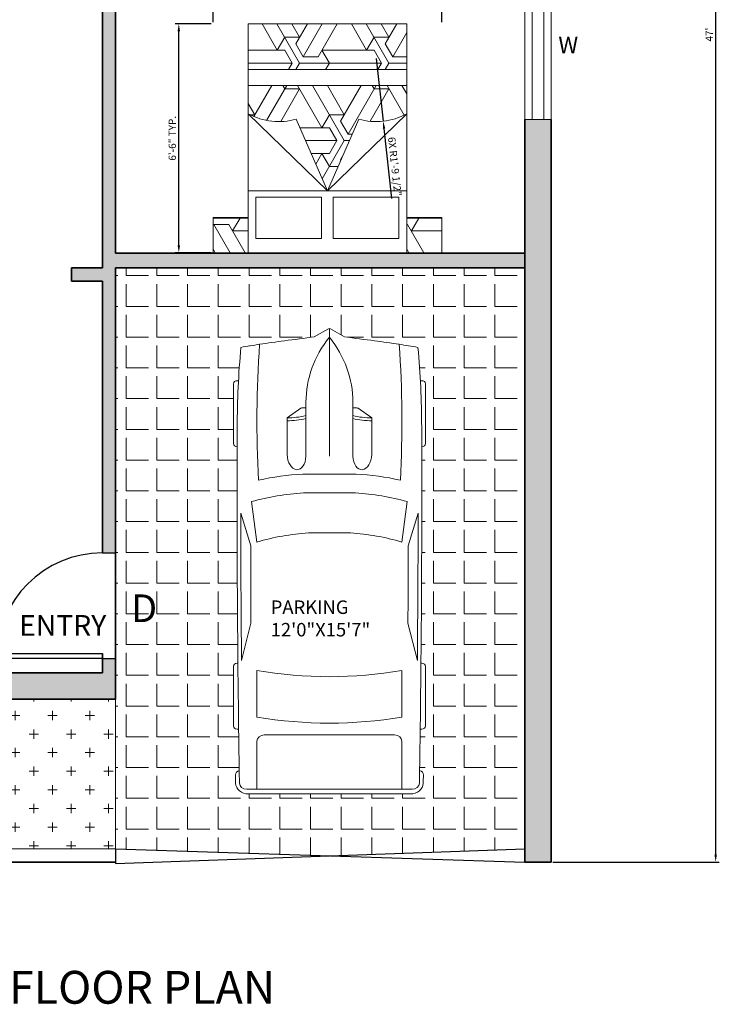
# Model space of a CAD drawing. Units: inches. Extents: x 1878 to 2382, y 1889 to 2524.
# Tile 1 of 2: x 2143 to 2382, y 1889 to 2225. Entities that reach past the tile are written whole.
import ezdxf

# ---------------------------------------------------------------- set-up
doc = ezdxf.new("R2010")
doc.units = ezdxf.units.IN
for name, color, linetype, lineweight in [('A-ANNO-DIMS', 2, 'Continuous', 18), ('A-ANNO-TEXT', 7, 'Continuous', 18), ('A-ANNO-TITL', 7, 'Continuous', 30), ('A-AREA-IDEN', 7, 'Continuous', 18), ('A-DOOR', 4, 'Continuous', 25), ('A-FLOR-PATT', 252, 'Continuous', 13), ('A-FURN', 8, 'Continuous', 18), ('A-FURN-PATT', 252, 'Continuous', 13), ('A-SITE-GATE', 1, 'Continuous', 25), ('A-SITE-VEHI', 8, 'Continuous', 18), ('A-WALL', 7, 'Continuous', 35), ('A-WALL-PATT', 251, 'Continuous', 13), ('L-PLNT', 3, 'Continuous', 18), ('L-PLNT-PATT', 3, 'Continuous', 13), ('windows', 5, 'Continuous', 18)]:
    doc.layers.add(name, color=color, linetype=linetype, lineweight=lineweight)
doc.styles.get("Standard").update_dxf_attribs({"font": 'arial.ttf'})
doc.dimstyles.new('ISO-25', dxfattribs={"dimtxt": 2.5, "dimasz": 2.5, "dimexe": 1.25, "dimexo": 0.625, "dimtad": 1, "dimlunit": 3, "dimtxsty": 'Standard', "dimcen": 2.5, "dimadec": 0, "dimazin": 0, "dimtfac": 1, "dimtmove": 0, "dimatfit": 3, "dimfxl": 1, "dimarcsym": 0})

# ---------------------------------------------------------------- blocks, each defined once
blk = doc.blocks.new('*D15')
at = {"layer": 'A-ANNO-DIMS', "color": 0, "lineweight": -2, "transparency": 16777216}
for p, q in [((2324.866440692248, 2501.568149098086), (2381.60236904706, 2501.568149098086)), ((2380.35236904706, 2499.068149098085), (2380.35236904706, 1940.068149098086)), ((2324.866440692248, 1937.568149098086), (2381.60236904706, 1937.568149098086))]:
    blk.add_line(p, q, dxfattribs=at)
at = {"layer": 'A-ANNO-DIMS', "color": 0, "transparency": 16777216}
for points in [[(2379.935702380393, 2499.068149098085), (2380.769035713727, 2499.068149098085), (2380.35236904706, 2501.568149098086)], [(2379.935702380393, 1940.068149098086), (2380.769035713727, 1940.068149098086), (2380.35236904706, 1937.568149098086)]]:
    blk.add_solid(points, dxfattribs=at)
at = {"layer": 'Defpoints', "color": 0, "transparency": 16777216}
for p in [(2324.241440692248, 2501.568149098086), (2324.241440692248, 1937.568149098086), (2380.35236904706, 1937.568149098086)]:
    blk.add_point(p, dxfattribs=at)
at = {"layer": 'A-ANNO-DIMS', "color": 0, "transparency": 16777216, "insert": (2378.47736904706, 2219.568149098085), "char_height": 2.5, "attachment_point": 5, "rotation": 90}
blk.add_mtext("47'", dxfattribs=at)
blk = doc.blocks.new('*U2')
for p, q in [((0, 0), (-1e-16, -3.999999999999999)), ((36, -4e-16), (36, -3.999999999999999))]:
    blk.add_line(p, q)
blk.add_lwpolyline([(0, 0), (5.2e-15, 36), (1.750000000000006, 36), (1.749999999999998, -7e-16)], close=True)
blk.add_arc((0, 0), 36, 0, 90)
blk = doc.blocks.new('*U17')
for p, q in [((21.10406751471477, 37.40863046792069), (21.10406751471477, 36.83230215753705)), ((46.55368679439944, 38.88847654282876), (22.35054758993934, 38.88847654282876)), ((47.80016686962392, 37.39011648242055), (47.80016686962392, 37.40863046792069)), ((87.98532186932616, 31.87120872459877), (74.75900729854769, 35.92175679182955)), ((135.4513231603356, 37.07354110333037), (135.4513231603356, 37.40863046792069)), ((136.6978032355602, 38.88847654282876), (160.90094244002, 38.88847654282867)), ((162.1474225152445, 37.40863046792049), (162.1474225152445, 36.77402019194128)), ((134.313356548143, 35.6043097713567), (119.2882629232503, 31.77757799177584)), ((186.4728846989705, -33.49860931502491), (186.4728846989718, 33.49860931502465)), ((188.3990091454065, -32.75868627757393), (188.3990091454077, 32.75868627757058)), ((70.0302824853563, 31.53613089391356), (86.40615155322342, 29.35124891408057)), ((138.4228833961707, 29.35124891408074), (157.2465674415997, 29.35124891408074)), ((186.4728846989718, 29.35124891408083), (167.0083537481071, 29.35124891408083)), ((164.515393597658, 26.39155676426461), (164.5153935976578, -26.39155676426503)), ((32.26591480791686, 11.62530558863241), (36.12873726252356, 17.16961494239206)), ((36.12873726252356, 17.16961494239206), (50.93891189819171, 17.16961494239206)), ((29.77279020470884, 9.505833383620029), (51.68362801571248, 9.505833383620029)), ((32.12291633764599, 9.505833383620029), (32.12291633764599, 11.15369945057711)), ((58.9167604809788, -10.77488335095668), (58.9167604809788, 10.77488335095617)), ((66.55009204259746, -10.5288681329018), (66.55009204259746, 10.52886813290129)), ((82.73706193978568, 8.496039918672748), (82.73706193978568, -8.49603991867258)), ((186.4728846989718, -10.5288681329018), (186.4728846989718, 10.52886813290129)), ((3.266462181856987, 6.128290093440767), (0.1022408397004821, 0.4060708604429806)), ((-4.43e-14, -2.558e-13), (51.68362801571248, -2.558e-13)), ((0.1022408397004821, -0.4060708604432933), (3.266462181856987, -6.128290093441194)), ((29.77279020470884, -9.50583338362054), (51.68362801571248, -9.50583338362054)), ((32.12291633764599, -9.50583338362054), (32.12291633764599, -11.15369945057762)), ((32.26591480791686, -11.62530558863292), (36.12873726252356, -17.16961494239257)), ((36.12873726252356, -17.16961494239257), (50.93891189819171, -17.16961494239257)), ((86.40615155322318, -29.35124891408145), (70.03028248535594, -31.53613089391442)), ((87.98532186932607, -31.87120872459903), (74.7590072985476, -35.92175679182964)), ((134.3133565481428, -35.60430977135721), (119.2882629232503, -31.77757799177618)), ((157.2465674415997, -29.35124891408117), (138.4228833961707, -29.35124891408126)), ((167.008353748107, -29.35124891408126), (186.4728846989707, -29.35124891408108)), ((21.10406751471477, -37.4086304679212), (21.10406751471477, -36.83230215753756)), ((46.55368679439944, -38.88847654282927), (22.35054758993934, -38.88847654282927)), ((47.80016686962392, -37.39011648242107), (47.80016686962392, -37.4086304679212)), ((135.4513231603355, -37.07354110333088), (135.4513231603355, -37.4086304679212)), ((136.6978032355602, -38.88847654282927), (160.9009424400199, -38.88847654282918)), ((162.1474225152445, -37.408630467921), (162.1474225152445, -36.77402019194179))]:
    blk.add_line(p, q)
for centre, major_axis, ratio, start_param, end_param in [((41.19115208863305, -490.8631038926156), (1.294e-13, 528.2339998381949), 0.8423038695439741, 0.0028100083536837, 0.0755983031096952), ((22.35054758993934, 37.40863046792072), (2.08e-14, -1.479846074908118), 0.842303869543976, 3.141592653589776, 4.712388980384677), ((64.48199294511879, -10555.61767587835), (1.907644e-10, 10593.02630634627), 0.842303869543847, -0.0133969486112073, 0.0027970409639888), ((46.55368679439944, 37.40863046792072), (2.2e-14, 1.479846074908118), 0.8423038695439758, -1.570796326794884, 1.73e-14), ((64.4819929449925, -10555.61767590795), (1.9177683e-09, -10591.54646030096), 0.8423038695482963, 3.133765086725325, 3.140440689641252), ((136.6978032355602, 37.40863046792072), (2.357e-13, -1.479846074908118), 0.842303869543976, 3.141592653589603, 4.712388980384554), ((160.90094244002, 37.40863046792052), (5.59e-14, 1.479846074908118), 0.842303869543976, -1.570796326794865, 4.44e-14), ((180.6280394947615, 35.8381667808375), (7.4e-14, 2.219769112362114), 0.8423038695439693, -0.0130174256259048, 1.249894140392862), ((64.48199294754608, -10556.35759891604), (1.349839377e-06, 10595.3130398087), 0.8423038681351469, -0.0133969484821159, -0.0130174254969711), ((183.9799245485226, 33.49860931502124), (3e-16, -2.959692149816168), 0.8423038695439952, 1.570796326796048, 3.128195704978389), ((183.9799245485216, 32.75868627756583), (8.56e-14, -5.246425615115243), 0.8423038695439737, 1.570796326795794, 3.128195704978164), ((266.0300214172791, -27.52442688366631), (1.966072e-10, 313.3077612809058), 0.8423038695435284, 1.367075990158062, 1.391760499156098), ((95.78879860270445, -3666.353346297651), (1.949864e-10, -3698.236159209632), 0.8423038695446962, 3.134048706297306, 3.14409775411291), ((259.1750197310735, -27.52442688366614), (1.506617e-10, -305.3028914627677), 0.8423038695443789, 4.528606069860317, 4.561837674556238), ((37.47375371777758, -593.9621830607928), (6.21e-14, -623.32820996736), 0.8423038695439826, 3.09604606856106, 3.200911180495224), ((134.4003789125686, 5.387441675477674), (4.276e-13, -89.7774543484738), 0.84230386954398, 4.44948196380473, 4.652344057257214), ((135.2911776514449, 5.387441675478555), (2.2715e-12, 81.77258453065997), 0.8423038695439563, 1.245306111696802, 1.507880129813836), ((149.595361812917, 2.799442537139299), (8.561e-13, -79.57966406425402), 0.842303869543983, 4.372215489277867, 4.640744122441986), ((17.08207736189386, -1.421e-13), (6.87e-14, 147.0179238898305), 0.8423038695439764, 4.511394369635731, 4.913383591133647), ((35.90576140732288, -1.421e-13), (6.87e-14, 147.0179238898305), 0.8423038695439764, 4.511394369635731, 4.913383591133647), ((167.0083537481071, 26.39155676426464), (1.394e-13, 2.959692149816236), 0.842303869543976, 5.55e-14, 1.57079632679492), ((-204.4946649195746, 52.39684969293512), (4.12053e-11, -250.9602162198571), 0.8423038695441164, 1.385369446298923, 1.434372047871027), ((13.03653510440275, 17.00972444508943), (1.2303e-12, 27.41599049210566), 0.8423038695439277, 4.435146050259648, 4.718221029521873), ((14.20086229321332, 17.00972444508943), (1.2303e-12, 27.41599049210566), 0.8423038695439277, 4.435146050259648, 4.718221029521873), ((50.7902773840875, 13.33772416300607), (6.340077547122382, -0.356608581037027), 0.6038335755719145, -1.39555193967809, 1.581314658479915), ((29.77279020470884, -46.66302566589627), (5.12e-14, 56.16885904951626), 0.842303869543976, 7e-16, 0.5903187773915901), ((32.74615637525823, 11.15369945057713), (1.313e-13, 0.7399230374541176), 0.8423038695439091, 0.8797135699495516, 1.570796326795045), ((0.6232400376122422, -1.421e-13), (1e-16, -0.7399230374541245), 0.842303869543842, 4.131459131953847, 5.293318828815531), ((29.77279020470884, 46.66302566589578), (4.004e-13, 56.16885904951626), 0.8423038695439734, 2.55127387619821, 3.141592653589801), ((-204.4946649195746, -52.39684969293552), (4.02945e-11, 250.9602162198562), 0.8423038695441192, -1.43437204787103, -1.385369446298926), ((32.74615637525823, -11.1536994505777), (1.3e-13, -0.7399230374541176), 0.8423038695439093, 4.712388980384541, 5.403471737230034), ((13.03653510440275, -17.00972444508983), (1.2568e-12, -27.41599049210552), 0.8423038695439318, 1.564964277657711, 1.848039256919935), ((14.20086229321332, -17.00972444508983), (1.2568e-12, -27.41599049210552), 0.8423038695439318, 1.564964277657711, 1.848039256919935), ((134.4003789125684, -5.387441675478584), (4.2949e-12, -89.77745434847827), 0.8423038695439354, -1.510751403667474, -1.307889310215002), ((135.2911776514465, -5.387441675480715), (3.2038e-12, -81.77258453066244), 0.8423038695439492, -1.50788012981387, -1.245306111696839), ((149.5953618129329, -2.799442537137565), (4.0897e-12, -79.57966406427697), 0.8423038695439419, -1.499151468852248, -1.230622835688196), ((259.1750197310694, 27.52442688365929), (1.08535e-11, 305.3028914629043), 0.8423038695439974, 1.721347632622872, 1.754579237318777), ((167.008353748107, -26.39155676426503), (1.02e-14, -2.959692149816192), 0.8423038695439885, 4.712388980384686, 6.283185307179581), ((266.0300214172791, 27.52442688366566), (8.75241e-11, 313.3077612806533), 0.8423038695441819, 1.749832154434603, 1.774516663432659), ((37.47375371777847, 593.9621830607904), (1.1693e-12, -623.3282099673584), 0.8423038695439528, -0.0593185269054384, 0.0455465850287298), ((95.78879860271888, 3666.35334629765), (1.637818e-10, -3698.236159209629), 0.8423038695447546, -0.0025051005232382, 0.007543947292366), ((41.19115208863322, 490.8631038926152), (1.37757e-11, -528.2339998381949), 0.8423038695440652, -0.0755983031097181, -0.0028100083537155), ((64.48199294503607, 10555.61767590793), (1.6049794e-09, -10591.54646030094), 0.8423038695397146, 0.0011519639481523, 0.0078275668641468), ((183.9799245485216, -33.4986093150211), (9.3e-15, 2.959692149816141), 0.8423038695439732, 3.154989602201626, 4.71238898038339), ((183.9799245485177, -32.7586862775633), (2.428e-13, -5.246425615118353), 0.8423038695439808, 0.0133969486110846, 1.570796326792831), ((22.35054758993934, -37.40863046792117), (2.2e-14, 1.479846074908118), 0.8423038695439758, 1.570796326794908, 3.14159265358981), ((64.48199294495228, 10555.61767590795), (6.117947e-10, 10593.02630637587), 0.8423038695458146, 3.138795612625926, 3.154989602201039), ((46.55368679439944, -37.40863046792117), (2.08e-14, -1.479846074908118), 0.842303869543976, -1.69e-14, 1.570796326794884), ((136.6978032355602, -37.40863046792109), (1.56e-14, -1.479846074908162), 0.8423038695440105, -1.570796326794875, -1.27e-14), ((160.9009424400199, -37.408630467921), (1.969e-13, 1.479846074908162), 0.8423038695440109, 3.141592653589951, 4.712388980384771), ((180.6280394947581, -35.83816678083949), (2.274e-13, -2.219769112363032), 0.8423038695439803, -1.249894138785958, 0.0130174256254374), ((64.48199294197605, 10556.3575989598), (9.365289701e-07, 10595.31303985772), 0.8423038705260315, 3.154610079306566, 3.154989602290631)]:
    blk.add_ellipse(centre, major_axis=major_axis, ratio=ratio, start_param=start_param, end_param=end_param)
at = {"extrusion": (0, 0, -1)}
blk.add_ellipse((50.7902773840875, -13.33772416300655), major_axis=(6.340077547122382, 0.3566085810370246), ratio=0.6038335755719145, start_param=-1.39555193967809, end_param=1.581314658479915, dxfattribs=at)
blk = doc.blocks.new('BED-DOUBLE-WITH-NIGHTSTANDS')
for p, q in [((39.00041612759128, 21.08000700798311), (12.00041612759128, 47.34561457886321)), ((39.00041612759128, 21.08000700798311), (66.00041612759127, 47.34561457886321)), ((39.00041612759128, 21.08000700798311), (28.35091833014235, 45.54110342781223)), ((39.00041612759128, 21.08000700798311), (49.64991392504021, 45.54110342781223)), ((66.00041612759127, 21.08000700798311), (12.00041612759128, 21.08000700798311)), ((36.91574546573361, 4.839445541926579), (36.91574546573361, 18.8744984206578)), ((40.91574546573361, 4.839445541926579), (40.91574546573361, 18.8744984206578)), ((0.0004161275912793, 0.0002775178572847), (0.0004161275912793, 12.00027751785728)), ((0.0004161275912793, 12.00027751785728), (12.00041612759128, 12.00027751785728)), ((78.00041612759128, 12.00027751785728), (66.00041612759127, 12.00027751785728)), ((78.00041612759128, 12.00027751785728), (78.00041612759128, 0.0002775178572847)), ((12.00041612759128, 0.0002775178572847), (0.0004161275912793, 0.0002775178572847)), ((66.00041612759127, 0.0002775178572847), (78.00041612759128, 0.0002775178572847))]:
    blk.add_line(p, q)
for points in [[(66.00041612759127, 78.00027751785728), (12.00041612759128, 78.00027751785728), (12.00041612759128, 0.0002775178572847), (66.00041612759127, 0.0002775178572847)], [(66.00041612759127, 56.96965028294471), (12.00041612759128, 56.96965028294471), (12.00041612759128, 62.38317077163083), (66.00041612759127, 62.38317077163083)]]:
    blk.add_lwpolyline(points, close=True)
for points in [[(36.91574546573361, 4.839445541926579), (14.53815381501522, 4.839445541926579), (14.53815381501522, 18.8744984206578), (36.91574546573361, 18.8744984206578)], [(40.91574546573361, 18.8744984206578), (63.29333711645199, 18.8744984206578), (63.29333711645199, 4.839445541926579), (40.91574546573361, 4.839445541926579)]]:
    blk.add_lwpolyline(points)
for centre, start, end in [((22.35293988504668, 66.17141739726458), 241.1931034301566, 286.2110586149389), ((55.64789237013588, 66.17141739726458), 253.7889413850611, 298.8068965698434)]:
    blk.add_arc(centre, 21.48454327897181, start, end)
blk = doc.blocks.new('WIN-51IN')
for p, q in [((4.500440692245319, 51.00020935019097), (0.0004406922455473, 51.00020935019074)), ((0.0004406922455473, 51.00020935019074), (9.000440692245093, 51.00020935019142)), ((0.0004406922482758, 0.0002093501907439), (0.0004406922441831, 51.00020935019074)), ((2.500440692248048, 0.0002093501907439), (2.500440692245319, 51.00020935019097)), ((6.500440692248048, 0.0002093501911986), (6.500440692245319, 51.0002093501912)), ((9.000440692245318, 51.0002093501912), (9.000440692247594, 0.0002093501911986)), ((0.0004406922482758, 0.0002093501907439), (9.000440692247821, 0.0002093501911986)), ((9.000440692247821, 0.0002093501911986), (4.500440692248048, 0.0002093501911986))]:
    blk.add_line(p, q)
blk = doc.blocks.new('*D21')
at = {"layer": 'A-ANNO-DIMS', "color": 0, "lineweight": -2, "transparency": 16777216}
for p, q in [((2208.998319239388, 2223.86759019772), (2208.998319239388, 2236.19259019772)), ((2211.498319239388, 2234.94259019772), (2284.498319239388, 2234.94259019772)), ((2286.998319239389, 2223.86759019772), (2286.998319239389, 2236.19259019772))]:
    blk.add_line(p, q, dxfattribs=at)
at = {"layer": 'A-ANNO-DIMS', "color": 0, "transparency": 16777216}
for points in [[(2211.498319239388, 2235.359256864387), (2211.498319239388, 2234.525923531053), (2208.998319239388, 2234.94259019772)], [(2284.498319239388, 2235.359256864387), (2284.498319239388, 2234.525923531053), (2286.998319239389, 2234.94259019772)]]:
    blk.add_solid(points, dxfattribs=at)
at = {"layer": 'Defpoints', "color": 0, "transparency": 16777216}
for p in [(2286.998319239389, 2234.94259019772), (2208.998319239388, 2223.24259019772), (2286.998319239389, 2223.24259019772)]:
    blk.add_point(p, dxfattribs=at)
at = {"layer": 'A-ANNO-DIMS', "color": 0, "transparency": 16777216, "insert": (2247.998319239389, 2236.860223212727), "char_height": 2.5, "attachment_point": 5}
blk.add_mtext('BED SET 6\'-6" TYP.', dxfattribs=at)
blk = doc.blocks.new('*D22')
at = {"layer": 'A-ANNO-DIMS', "color": 0, "lineweight": -2, "transparency": 16777216}
for p, q in [((2208.373319239389, 2223.242590197721), (2196.048319239391, 2223.242590197721)), ((2197.29831923939, 2147.742590197721), (2197.29831923939, 2220.742590197721)), ((2208.373319239389, 2145.242590197721), (2196.048319239391, 2145.242590197721))]:
    blk.add_line(p, q, dxfattribs=at)
at = {"layer": 'A-ANNO-DIMS', "color": 0, "transparency": 16777216}
for points in [[(2196.881652572724, 2220.742590197721), (2197.714985906057, 2220.742590197721), (2197.29831923939, 2223.242590197721)], [(2196.881652572724, 2147.742590197721), (2197.714985906057, 2147.742590197721), (2197.29831923939, 2145.242590197721)]]:
    blk.add_solid(points, dxfattribs=at)
at = {"layer": 'Defpoints', "color": 0, "transparency": 16777216}
for p in [(2197.29831923939, 2223.242590197721), (2208.998319239389, 2223.242590197721), (2208.998319239389, 2145.242590197721)]:
    blk.add_point(p, dxfattribs=at)
at = {"layer": 'A-ANNO-DIMS', "color": 0, "transparency": 16777216, "insert": (2195.396886770086, 2184.242590197721), "char_height": 2.5, "attachment_point": 5, "rotation": 90}
blk.add_mtext('6\'-6" TYP.', dxfattribs=at)
blk = doc.blocks.new('*D28')
at = {"layer": 'A-ANNO-DIMS', "color": 0, "lineweight": -2, "transparency": 16777216}
for p, q in [((2264.645795, 2211.41373), (2266.999068, 2190.058457000001)), ((2269.901588536305, 2163.71892119566), (2267.272901265089, 2187.57349918488))]:
    blk.add_line(p, q, dxfattribs=at)
at = {"layer": 'A-ANNO-DIMS', "color": 0, "transparency": 16777216}
blk.add_solid([(2267.687060900943, 2187.619138062395), (2266.858741629236, 2187.527860307365), (2266.999068, 2190.058457000001)], dxfattribs=at)
at = {"layer": 'Defpoints', "color": 0, "transparency": 16777216}
for p in [(2264.645795, 2211.41373), (2266.999068, 2190.058457000001)]:
    blk.add_point(p, dxfattribs=at)
at = {"layer": 'A-ANNO-DIMS', "color": 0, "transparency": 16777216, "insert": (2270.630256392112, 2174.613775966606), "char_height": 2.5, "attachment_point": 5, "rotation": 276.2884134152478}
blk.add_mtext('6X R1\'-9 1/2"', dxfattribs=at)

msp = doc.modelspace()

# ---------------------------------------------------------------- hatches: boundary and pattern name
at = {"layer": 'A-FLOR-PATT'}
h = msp.add_hatch(dxfattribs=at)
h.set_pattern_fill('ANGLE', color=256, scale=1.5)
h.set_pattern_definition([(0, (0, 0), (0, 10.4775), [7.62, -2.857499999999999]), (90, (0, 0), (-10.4775, 6e-16), [7.62, -2.857499999999999])])
h.paths.add_polyline_path([(2315.241440692247, 2140.068149098084), (2175.741440692247, 2140.068149098084), (2175.741440692247, 1993.068149098084), (2175.741440692247, 1942.068149098084), (2248.893126853422, 1939.708417286433), (2315.241440692247, 1942.068149098084), (2315.241440692247, 1946.568149098084)])
edge = h.paths.add_edge_path(flags=16)
edge.add_ellipse((2217.163435380962, 2100.560026434194), major_axis=(1.245847997764485, 6.167e-13), ratio=0.8423038695438281, start_angle=89.99999999997169, end_angle=179.9999999999717, ccw=False)
edge.add_line((2217.163435380962, 2101.609409023574), (2217.648632783395, 2101.609409023574))
edge.add_ellipse((2661.903123979704, 2084.698559630743), major_axis=(444.7079207818702, 3.18231e-11), ratio=0.8423038695442732, start_angle=176.3495724142969, end_angle=177.8200496863507, ccw=False)
edge.add_ellipse((2271.829066396155, 1895.411944000707), major_axis=(263.7665184880922, 8.500711e-10), ratio=0.8423038695417554, start_angle=102.12596555209939, end_angle=103.78052898931321, ccw=False)
edge.add_ellipse((2271.829066396149, 1901.18301051245), major_axis=(257.0274047359001, 9.496292e-10), ratio=0.8423038695409001, start_angle=100.20953899693149, end_angle=102.44462729323232, ccw=False)
edge.add_ellipse((2204.545202155118, 2291.53573573221), major_axis=(-211.2775701453485, 2.757678e-10), ratio=0.8423038695450628, start_angle=99.2565660072763, end_angle=102.554932644212)
edge.add_line((2243.497626541594, 2116.626474153294), (2248.417311037811, 2119.346917052413))
edge.add_ellipse((2248.656891462514, 2118.851741410404), major_axis=(-0.6229239988830404, 7.883e-13), ratio=0.8423038695431149, start_angle=270.00000000007253, end_angle=307.93313045992204, ccw=False)
edge.add_ellipse((2248.656891462514, 2118.851741410404), major_axis=(-0.6229239988830404, 7.883e-13), ratio=0.8423038695431149, start_angle=232.06686954025992, end_angle=270.00000000007253, ccw=False)
edge.add_line((2248.99875307705, 2119.290358519684), (2253.816156383433, 2116.626474153294))
edge.add_ellipse((2292.76858076991, 2291.53573573221), major_axis=(211.2775701452792, 3.37693e-10), ratio=0.8423038695453325, start_angle=257.4450673557711, end_angle=260.7434339927067)
edge.add_ellipse((2225.484716528872, 1901.183010512447), major_axis=(-257.027404735798, 8.224738e-10), ratio=0.8423038695412367, start_angle=257.5553727067381, end_angle=259.7904610030389, ccw=False)
edge.add_ellipse((2225.484716528872, 1895.411944000707), major_axis=(-263.7665184880879, 8.429844e-10), ratio=0.842303869541768, start_angle=256.2194710106853, end_angle=257.87403444789913, ccw=False)
edge.add_ellipse((1835.410658945323, 2084.698559630743), major_axis=(444.7079207818702, 4.84123e-11), ratio=0.842303869543595, start_angle=2.179950313638926, end_angle=3.650427585692796, ccw=False)
edge.add_line((2279.665150141632, 2101.609409023574), (2280.150347544065, 2101.609409023574))
edge.add_ellipse((2280.150347544065, 2100.560026434194), major_axis=(1.245847997764485, 1.2485e-12), ratio=0.8423038695438281, start_angle=-5.7411853049416095e-11, end_angle=89.99999999994259, ccw=False)
edge.add_line((2281.39619554183, 2100.560026434194), (2281.39619554183, 2080.183966363644))
edge.add_ellipse((2280.150347544065, 2080.183966363644), major_axis=(-1.245847997764485, 1.2482e-12), ratio=0.8423038695438281, start_angle=90.00000000005741, end_angle=180.0000000000574, ccw=False)
edge.add_ellipse((-6637.872166958759, 2065.090542324547), major_axis=(-8918.022514502822, 3.054967e-10), ratio=0.8423038695434657, start_angle=179.6161332212095, end_angle=180.0902290885963, ccw=False)
edge.add_line((2279.868243600263, 2005.34311355442), (2280.150347544065, 2005.34311355442))
edge.add_ellipse((2280.150347544065, 2004.293730965039), major_axis=(1.245847997764485, 7.899e-13), ratio=0.8423038695441931, start_angle=-3.632294465205632e-11, end_angle=89.99999999996368, ccw=False)
edge.add_line((2281.39619554183, 2004.293730965039), (2281.39619554183, 1983.91767089449))
edge.add_ellipse((2280.150347544065, 1983.91767089449), major_axis=(1.24584799776494, 8.529e-13), ratio=0.8423038695437032, start_angle=269.9999999999607, end_angle=359.9999999999608, ccw=False)
edge.add_line((2280.150347544065, 1982.868288305109), (2279.616083910097, 1982.868288305109))
edge.add_ellipse((-6637.872166958759, 2065.090542324547), major_axis=(-8918.022514502822, 3.054967e-10), ratio=0.8423038695434657, start_angle=179.3813568036828, end_angle=179.471728528184, ccw=False)
edge.add_ellipse((2278.828210685854, 1967.309886622816), major_axis=(-1.868771996646647, 2.868e-13), ratio=0.8423038695439512, start_angle=179.3717627838123, end_angle=248.46475660101112, ccw=False)
edge.add_ellipse((-6638.495090957841, 2065.090542322504), major_axis=(-8919.947662225442, 2.5216408041e-06), ratio=0.8423038664257816, start_angle=179.3534459191486, end_angle=179.3717627999817, ccw=False)
edge.add_ellipse((2276.235667661138, 1964.488012541606), major_axis=(4.416843723708598, 7.672e-13), ratio=0.8423038695439437, start_angle=-89.9999999999468, end_angle=-0.64655409709178, ccw=False)
edge.add_line((2276.235667661142, 1960.767687981955), (2221.078115263882, 1960.767687981956))
edge.add_ellipse((2221.078115263891, 1964.488012541609), major_axis=(4.416843723710838, 1.258e-13), ratio=0.84230386954398, start_angle=180.6465540970563, end_angle=269.99999999985835, ccw=False)
edge.add_ellipse((11135.80887391971, 2065.090542327189), major_axis=(-8919.947662268243, 7.86809242e-08), ratio=0.8423038696526933, start_angle=0.6282372167484027, end_angle=0.6465540975815998, ccw=False)
edge.add_ellipse((2218.485572239172, 1967.309886622819), major_axis=(1.868771996647995, 1.7504e-12), ratio=0.8423038695439624, start_angle=111.5352435039834, end_angle=180.6282372161214, ccw=False)
edge.add_ellipse((11135.1859499087, 2065.090542324684), major_axis=(-8918.022514527744, 3.035165e-10), ratio=0.8423038695434527, start_angle=0.5282714718193233, end_angle=0.6465540970629036, ccw=False)
edge.add_line((2217.69769901493, 1982.868288305109), (2217.163435380962, 1982.868288305109))
edge.add_ellipse((2217.163435380962, 1983.91767089449), major_axis=(-1.24584799776494, 1.6355e-12), ratio=0.8423038695438858, start_angle=7.5203843152849e-11, end_angle=90.00000000007509, ccw=False)
edge.add_line((2215.917587383197, 1983.91767089449), (2215.917587383197, 2004.293730965039))
edge.add_ellipse((2217.163435380962, 2004.293730965039), major_axis=(1.24584799776494, 5.287e-13), ratio=0.8423038695438858, start_angle=90.00000000000051, end_angle=179.9999999999757, ccw=False)
edge.add_line((2217.163435380962, 2005.34311355442), (2217.445539324763, 2005.34311355442))
edge.add_ellipse((11135.1859499087, 2065.090542324684), major_axis=(-8918.022514527744, 3.035165e-10), ratio=0.8423038695434527, start_angle=-0.09022908859117251, end_angle=0.38386677879429953, ccw=False)
edge.add_ellipse((2217.163435380962, 2080.183966363644), major_axis=(-1.245847997764485, 6.167e-13), ratio=0.8423038695438281, start_angle=2.8421709430404007e-11, end_angle=90.00000000002842, ccw=False)
edge.add_line((2215.917587383197, 2080.183966363644), (2215.917587383197, 2100.560026434194))
edge = h.paths.add_edge_path(flags=0)
edge.add_line((2234.202191908915, 2088.960488950219), (2238.869817025127, 2092.212509347739))
edge.add_ellipse((2239.266851265912, 2091.808205139849), major_axis=(0.6229239988828434, 1.5188e-12), ratio=0.8423038695433808, start_angle=89.99999999986028, end_angle=134.4802108824004, ccw=False)
edge.add_line((2239.266851265912, 2092.332896434539), (2240.654151387805, 2092.332896434539))
edge.add_line((2240.654151387805, 2092.332896434539), (2240.654151387805, 2094.311412975454))
edge.add_ellipse((2287.941407657283, 2094.311412975454), major_axis=(-47.28725626947833, 4.4023e-12), ratio=0.8423038695439483, start_angle=-29.43856959797438, end_angle=5.286437954055145e-12, ccw=False)
edge.add_ellipse((2209.372375267744, 2094.311412975454), major_axis=(47.28725626947835, 1.4099e-12), ratio=0.8423038695439753, start_angle=-1.7053025658242404e-12, end_angle=29.438569597978073, ccw=False)
edge.add_line((2256.659631537222, 2094.311412975454), (2256.659631537222, 2092.332896434539))
edge.add_line((2256.659631537222, 2092.332896434539), (2258.046931659115, 2092.332896434539))
edge.add_ellipse((2258.046931659115, 2091.808205139849), major_axis=(-0.6229239988828434, 1.5188e-12), ratio=0.842303869543381, start_angle=225.5197891175996, end_angle=270.00000000013966, ccw=False)
edge.add_line((2258.4439658999, 2092.212509347739), (2263.111591016112, 2088.960488950219))
edge.add_line((2263.111591016112, 2088.960488950219), (2263.111591016112, 2076.492147323853))
edge.add_ellipse((2259.885611276667, 2076.617279264894), major_axis=(0.3002204717125075, 5.337563853217266), ratio=0.6038335755718899, start_angle=106.3425919543044, end_angle=270.99798572497696, ccw=False)
edge.add_line((2256.659631537222, 2075.865188142322), (2256.659631537222, 2094.311412975454))
edge.add_ellipse((2209.372375267744, 2094.311412975454), major_axis=(47.28725626947835, 1.4099e-12), ratio=0.8423038695439753, start_angle=-1.7038e-12, end_angle=29.43856959797809)
edge.add_ellipse((2287.941407657283, 2094.311412975454), major_axis=(-47.28725626947833, 4.4023e-12), ratio=0.8423038695439483, start_angle=-29.43856959797446, end_angle=5.3258e-12)
edge.add_line((2240.654151387805, 2094.311412975454), (2240.654151387805, 2075.865188142322))
edge.add_ellipse((2237.42817164836, 2076.617279264894), major_axis=(-0.3002204717125075, 5.337563853217266), ratio=0.6038335755718899, start_angle=89.0020142750231, end_angle=253.6574080456956, ccw=False)
edge.add_line((2234.202191908915, 2076.492147323853), (2234.202191908915, 2088.960488950219))
edge = h.paths.add_edge_path(flags=0)
edge.add_ellipse((2244.121329596806, 2005.477936334291), major_axis=(68.84243735681609, 2.73816e-11), ratio=0.8423038695437094, start_angle=94.27742096303137, end_angle=111.8349537966854, ccw=False)
edge.add_line((2239.792882222284, 2063.349457786458), (2257.520900702743, 2063.349457786458))
edge.add_ellipse((2253.19245332822, 2005.477936334292), major_axis=(-68.84243735680111, 1.27834e-11), ratio=0.8423038695438707, start_angle=248.1650462033007, end_angle=265.72257903695515, ccw=False)
edge.add_line((2275.206426713241, 2060.419566381894), (2273.367025382197, 2046.633103022099))
edge.add_ellipse((2251.013677035613, 1993.435576321726), major_axis=(66.99626861082456, 8.2306e-12), ratio=0.8423038695440823, start_angle=67.20808512240309, end_angle=85.12993040285708)
edge.add_line((2255.809509901066, 2049.72202424575), (2241.504273023962, 2049.72202424575))
edge.add_ellipse((2246.300105889415, 1993.435576321713), major_axis=(-66.99626861084705, 1.0603e-12), ratio=0.8423038695440016, start_angle=-85.12993040286347, end_angle=-67.2080851224124)
edge.add_line((2223.946757542829, 2046.633103022099), (2222.107356211785, 2060.419566381894))
edge = h.paths.add_edge_path(flags=0)
edge.add_line((2218.415199752743, 2056.438562924582), (2221.825261978115, 2045.303636255376))
edge.add_ellipse((5335.274515438081, 2038.734070657485), major_axis=(3113.459022755477, 1.370733e-10), ratio=0.842303869546709, start_angle=179.8791026309645, end_angle=180.3640763488875)
edge.add_line((2221.904087514766, 2018.950418108292), (2218.682451017289, 2006.30114118268))
edge.add_ellipse((11135.18594990869, 2065.090542324613), major_axis=(-8916.776666529968, 7.271774e-10), ratio=0.8423038695453231, start_angle=0.05559431350371824, end_angle=0.3777641939141745, ccw=False)
edge = h.paths.add_edge_path(flags=0)
edge.add_ellipse((-6637.872166983679, 2065.090542324654), major_axis=(8916.77666652998, 1.2280977e-09), ratio=0.8423038695482251, start_angle=-0.37776419391781246, end_angle=-0.055594313507299375, ccw=False)
edge.add_line((2278.631331907739, 2006.301141182676), (2275.409695410262, 2018.950418108291))
edge.add_ellipse((-837.9607325130555, 2038.734070657497), major_axis=(3113.45902275548, 2.850173e-10), ratio=0.8423038695464728, start_angle=-0.3640763488955833, end_angle=0.1208973690274228)
edge.add_line((2275.488520946915, 2045.303636255384), (2278.898583172285, 2056.438562924586))
edge = h.paths.add_edge_path(flags=0)
edge.add_ellipse((2248.656891462514, 2104.995429004897), major_axis=(-123.7709713322896, 1.1069e-12), ratio=0.8423038695439762, start_angle=76.40186530976968, end_angle=103.598134690231)
edge.add_line((2273.367025382198, 2002.841426093254), (2273.367025382198, 1986.994204225934))
edge.add_ellipse((2248.656891462514, 2089.148207137577), major_axis=(123.770971332293, 6.397e-13), ratio=0.8423038695439492, start_angle=256.4018653097689, end_angle=283.59813469023027, ccw=False)
edge.add_line((2223.946757542829, 1986.994204225935), (2223.946757542829, 2002.841426093254))
edge = h.paths.add_edge_path(flags=0)
edge.add_ellipse((2226.438453538359, 1978.775983337439), major_axis=(2.491695995529425, 3.863e-13), ratio=0.842303869543857, start_angle=89.99999999999119, end_angle=179.9999999999912, ccw=False)
edge.add_line((2226.438453538359, 1980.874748516201), (2270.875329386669, 1980.874748516201))
edge.add_ellipse((2270.875329386668, 1978.775983337439), major_axis=(-2.491695995529425, 3.858e-13), ratio=0.842303869543857, start_angle=180.0000000000089, end_angle=269.9999999999964, ccw=False)
edge.add_line((2273.367025382198, 1978.775983337439), (2273.367025382198, 1962.389247362843))
edge.add_line((2273.367025382198, 1962.389247362843), (2223.94675754283, 1962.389247362844))
edge.add_line((2223.94675754283, 1962.389247362844), (2223.946757542829, 1978.775983337439))
h.paths.add_polyline_path([(2226.77806988673, 2011.848788610063), (2261.830806516837, 2011.848788610063), (2261.830806516837, 2029.016856799895), (2226.77806988673, 2029.016856799895)], flags=8)
at = {"layer": 'A-FURN-PATT'}
h = msp.add_hatch(dxfattribs=at)
h.set_pattern_fill('ESCHER', color=256, angle=180)
h.set_pattern_definition([(240, (4646.383709742781, 4638.30217860601), (30.47999998809242, 6.8748365e-09), [27.94, -2.539999999999999]), (360, (4646.383709742781, 4638.30217860601), (-15.23999999999999, 26.39645429360001), [27.94, -2.54]), (120, (4646.383709742781, 4638.30217860601), (-30.47999998809242, 6.874844e-09), [27.94, -2.539999999999999]), (240, (4643.843709742781, 4638.30217860601), (30.47999998809242, 6.8748365e-09), [5.079999999999999, -25.4]), (120, (4643.843709742781, 4638.30217860601), (-30.47999998809242, 6.874844e-09), [5.079999999999999, -25.4]), (240, (4647.653709742781, 4636.102474090011), (30.47999998809242, 6.8748365e-09), [5.079999999999999, -25.4]), (360, (4647.653709742781, 4636.102474090011), (-15.23999999999999, 26.39645429360001), [5.08, -25.4]), (120, (4647.653709742781, 4640.50188312201), (-30.47999998809242, 6.874844e-09), [5.079999999999999, -25.4]), (360, (4647.653709742781, 4640.50188312201), (-15.23999999999999, 26.39645429360001), [5.08, -25.4]), (240, (4656.54370974278, 4638.30217860601), (30.47999998809242, 6.8748365e-09), [5.079999999999999, -25.4]), (120, (4656.54370974278, 4638.30217860601), (-30.47999998809242, 6.874844e-09), [5.079999999999999, -25.4]), (240, (4641.30370974278, 4647.10099669541), (30.47999998809242, 6.8748365e-09), [5.079999999999999, -25.4]), (360, (4641.30370974278, 4647.10099669541), (-15.23999999999999, 26.39645429360001), [5.08, -25.4]), (120, (4641.30370974278, 4629.50336051661), (-30.47999998809242, 6.874844e-09), [5.079999999999999, -25.4]), (360, (4641.30370974278, 4629.50336051661), (-15.23999999999999, 26.39645429360001), [5.08, -25.4]), (180, (4641.30370974278, 4633.902769548611), (15.24, -26.39645429360001), [17.78, -12.7]), (180, (4641.30370974278, 4642.701587663411), (15.24, -26.39645429360001), [17.78, -12.7]), (300, (4645.11370974278, 4631.70306503261), (30.47999998809242, -6.8748546e-09), [17.77999999999999, -12.69999999999999]), (300, (4652.733709742781, 4636.102474090011), (30.47999998809242, -6.8748546e-09), [17.77999999999999, -12.69999999999999]), (59.99999999999997, (4652.733709742781, 4640.50188312201), (-15.2399999880924, 26.39645430047486), [17.78, -12.7]), (59.99999999999997, (4645.11370974278, 4644.901292179411), (-15.2399999880924, 26.39645430047486), [17.78, -12.7])])
h.paths.add_polyline_path([(2247.998319239388, 2166.322319687846), (2258.647817036837, 2190.783416107675, 0.1989938127017897), (2274.998319239388, 2192.587927258726), (2274.998319239388, 2202.211962962807), (2220.998319239388, 2202.211962962807), (2220.998319239388, 2192.587927258726, 0.1989938127017895), (2237.348821441939, 2190.783416107675)])
h.paths.add_polyline_path([(2274.998319239388, 2207.625483451494), (2274.998319239388, 2223.24259019772), (2220.998319239388, 2223.24259019772), (2220.998319239388, 2207.625483451494)])
h.paths.add_polyline_path([(2208.998319239388, 2157.24259019772), (2208.998319239388, 2145.24259019772), (2220.998319239388, 2145.24259019772), (2220.998319239388, 2157.24259019772)])
h.paths.add_polyline_path([(2286.998319239388, 2157.24259019772), (2274.998319239388, 2157.24259019772), (2274.998319239388, 2145.24259019772), (2286.998319239388, 2145.24259019772)])
at = {"layer": 'A-WALL-PATT'}
h = msp.add_hatch(color=256, dxfattribs=at)
h.dxf.hatch_style = 1
h.paths.add_polyline_path([(1925.241440692247, 2376.261341107433), (1916.241440692247, 2376.261341107433), (1916.241440692247, 2322.068149098084), (1920.741440692247, 2322.068149098084), (1925.241440692247, 2322.068149098084)])
h.paths.add_polyline_path([(1925.241440692247, 2286.140121582637), (1916.241440692247, 2286.068149098084), (1916.241440692247, 2097.50720935019), (1920.741440692247, 2097.50720935019), (1925.241440692246, 2097.50720935019)])
h.paths.add_polyline_path([(1925.241440692246, 2046.50720935019), (1916.241440692247, 2046.50720935019), (1916.241440692247, 1993.068149098084), (1925.241440692247, 1993.068149098084), (2100.228537208572, 1993.068149098084), (2100.228537208572, 1997.568149098084), (2100.228537208572, 2002.068149098084), (2052.741440692247, 2002.068149098084), (2052.741440692247, 2135.568149098084), (2048.241440692248, 2135.568149098084), (2048.241440692248, 2002.068149098084), (1925.241440692246, 2002.068149098084)])
h.paths.add_polyline_path([(2175.741440692247, 2006.934770096195), (2175.253494205439, 2006.934770096195), (2171.241440692247, 2006.934770096195), (2171.241440692247, 2002.068149098084), (2136.228537208572, 2002.068149098084), (2136.228537208572, 1993.068149098084), (2171.241440692247, 1993.068149098084), (2175.741440692247, 1993.068149098084)])
h.paths.add_polyline_path([(1925.241440692247, 2492.568149098084), (2018.709393843749, 2492.568149098085), (2018.709393843749, 2497.068149098084), (2018.709393843749, 2501.568149098084), (1916.241440692247, 2501.568149098084), (1916.241440692247, 2427.261341107433), (1925.241440692247, 2427.261341107433)])
h.paths.add_polyline_path([(2324.241440692247, 2501.568149098084), (2052.741440692247, 2501.568149098084), (2052.741440692247, 2497.068149098084), (2319.741440692247, 2497.068149098084), (2319.741440692247, 2446.568149098084), (2324.241440692247, 2446.568149098084)])
h.paths.add_polyline_path([(2110.637963685758, 2446.568149098085), (2052.741440692248, 2446.568149098085), (2052.741440692247, 2492.568149098085), (2048.241440692248, 2492.568149098085), (2048.241440692248, 2446.568149098084), (1976.241440692247, 2446.568149098084), (1976.241440692247, 2442.068149098084), (2048.241440692248, 2442.068149098084), (2048.241440692248, 2326.568149098084), (2052.741440692248, 2326.568149098084), (2052.741440692248, 2442.068149098085), (2110.637963685758, 2442.068149098085), (2110.637963685758, 2444.318149098084)])
h.paths.add_polyline_path([(2100.741440692248, 2326.568149098084), (2052.741440692248, 2326.568149098084), (2052.741440692248, 2322.068149098084), (2100.741440692248, 2322.068149098084)])
h.paths.add_polyline_path([(2052.741440692248, 2326.568149098084), (2048.241440692248, 2326.568149098084), (2048.241440692248, 2322.068149098084), (2052.741440692248, 2322.068149098084)])
h.paths.add_polyline_path([(2048.241440692248, 2326.568149098084), (2045.469072311536, 2326.568149098084), (2045.469072311536, 2326.564566759995), (2045.469072311536, 2322.564566759995), (2045.469072311536, 2322.068149098084), (2048.241440692248, 2322.068149098084)])
h.paths.add_polyline_path([(2009.469072311536, 2326.568149098084), (1925.241440692247, 2326.568149098084), (1925.241440692247, 2322.068149098084), (2009.469072311536, 2322.068149098084), (2009.469072311536, 2322.564566759995)])
h.paths.add_polyline_path([(2315.241440692247, 2326.568149098084), (2259.241440692248, 2326.568149098084), (2259.241440692247, 2405.455505715361), (2255.232373025363, 2405.455505715361), (2254.741440692247, 2405.455505715361), (2254.741440692247, 2326.568149098084), (2207.241440692247, 2326.568149098084), (2195.241440692247, 2326.568149098084), (2195.241440692247, 2322.068149098084), (2207.241440692247, 2322.068149098084), (2207.241440692247, 2317.983016143046), (2207.736123013865, 2317.983016143046), (2211.741440692247, 2317.983016143046), (2211.741440692247, 2322.068149098084), (2315.241440692247, 2322.068149098084)])
h.paths.add_polyline_path([(2315.241440692247, 2446.568149098084), (2161.637963685759, 2446.568149098084), (2161.637963685759, 2442.068149098084), (2254.741440692248, 2442.068149098084), (2254.741440692248, 2435.45550571536), (2255.232373025363, 2435.45550571536), (2259.241440692247, 2435.45550571536), (2259.241440692247, 2442.068149098084), (2315.241440692247, 2442.068149098084)])
h.paths.add_polyline_path([(2315.241440692247, 2274.068149098084), (2207.241440692247, 2274.068149098084), (2171.241440692247, 2274.068149098084), (2171.241440692247, 2265.326277142973), (2171.730927479741, 2265.326277142973), (2175.741440692247, 2265.326277142973), (2175.741440692247, 2269.568149098084), (2315.241440692247, 2269.568149098084)])
h.paths.add_polyline_path([(2226.77806988673, 2011.848788610063), (2261.830806516837, 2011.848788610063), (2261.830806516837, 2029.016856799895), (2226.77806988673, 2029.016856799895)], flags=9)
h.paths.add_polyline_path([(2187.32039703604, 2282.173908487125), (2191.179537554457, 2282.173908487125), (2191.179537554457, 2287.32568202055), (2187.32039703604, 2287.32568202055)], flags=9)
h.paths.add_polyline_path([(2140.303776002406, 2010.813127097478), (2177.357239682197, 2010.813127097478), (2177.357239682197, 2025.39985028964), (2140.303776002406, 2025.39985028964)], flags=9)
h.paths.add_polyline_path([(2106.34299009357, 2361.376149589321), (2203.937232242951, 2361.376149589321), (2203.937232242951, 2388.800664716006), (2106.34299009357, 2388.800664716006)], flags=9)
h.paths.add_polyline_path([(2229.025427119923, 2239.685701226347), (2287.845526911306, 2239.685701226347), (2287.845526911306, 2264.045270653161), (2229.025427119923, 2264.045270653161)], flags=9)
h.paths.add_polyline_path([(2039.469638618838, 2246.05759564136), (2106.461015502027, 2246.05759564136), (2106.461015502027, 2270.434976204787), (2039.469638618838, 2270.434976204787)], flags=9)
h.paths.add_polyline_path([(2080.263524544797, 2072.342763218177), (2149.799479349807, 2072.342763218177), (2149.799479349807, 2093.991209603414), (2080.263524544797, 2093.991209603414)], flags=9)
h = msp.add_hatch(color=256, dxfattribs=at)
h.dxf.hatch_style = 1
h.paths.add_polyline_path([(2324.241440692247, 2283.876461182277), (2315.241440692247, 2283.876461182277), (2315.241440692247, 2241.595705025093), (2324.241440692247, 2241.595705025093)])
h.paths.add_polyline_path([(2324.241440692247, 2190.595705025093), (2315.241440692247, 2190.595705025093), (2315.241440692247, 1946.568149098084), (2315.241440692247, 1937.568149098084), (2324.241440692247, 1937.568149098084)])
h.paths.add_polyline_path([(2315.241440692247, 2145.068149098084), (2175.741440692247, 2145.068149098084), (2175.741440692247, 2229.326277142973), (2171.730927479741, 2229.326277142973), (2171.241440692247, 2229.326277142973), (2171.241440692247, 2145.068149098084), (2171.241440692247, 2140.568149098085), (2171.241440692247, 2140.068149098084), (2160.741440692248, 2140.068149098084), (2160.741440692248, 2135.568149098084), (2171.241440692247, 2135.568149098084), (2171.241440692247, 2042.934770096195), (2175.253494205439, 2042.934770096195), (2175.741440692247, 2042.934770096195), (2175.741440692247, 2140.068149098084), (2315.241440692247, 2140.068149098084)])
at = {"layer": 'L-PLNT-PATT'}
h = msp.add_hatch(dxfattribs=at)
h.set_pattern_fill('CROSS', color=256)
h.set_pattern_definition([(0, (0, 0), (6.349999999999999, 6.349999999999999), [3.174999999999999, -9.525]), (90, (1.587499999999999, -1.587499999999999), (-6.349999999999999, 6.349999999999999), [3.174999999999999, -9.525])])
h.paths.add_polyline_path([(2175.741440692247, 1942.068149098084), (2175.741440692247, 1993.068149098084), (2171.241440692247, 1993.068149098084), (2136.228537208572, 1993.068149098084), (2100.228537208572, 1993.068149098084), (1925.241440692247, 1993.068149098084), (1920.741440692247, 1993.068149098084), (1920.741440692247, 1942.068149098084)])

# ---------------------------------------------------------------- linework, layer by layer
at = {"layer": 'A-DOOR'}
for p, q in [((2175.253494205439, 2042.934770096195), (2175.741440692247, 2042.934770096195)), ((2175.253494205439, 2006.934770096195), (2175.741440692247, 2006.934770096195))]:
    msp.add_line(p, q, dxfattribs=at)
at = {"layer": 'A-SITE-GATE'}
for p, q in [((2175.741440692247, 1942.068149098084), (2175.741440692247, 1937.106717997892)), ((2175.741440692247, 1937.106717997892), (2315.241440692247, 1942.068149098084)), ((2175.741440692247, 1942.068149098084), (2315.241440692247, 1937.568149098084))]:
    msp.add_line(p, q, dxfattribs=at)
at = {"layer": 'A-WALL'}
for p, q in [((2171.241440692247, 2145.068149098084), (2171.241440692247, 2274.068149098084)), ((2175.741440692247, 2145.068149098084), (2175.741440692247, 2229.32627867808)), ((2315.241440692247, 2190.595705025093), (2315.241440692247, 1946.568149098084)), ((2324.241440692247, 2190.595705025093), (2324.241440692247, 1937.568149098084)), ((2171.241440692247, 2140.568149098085), (2171.241440692247, 2145.068149098084)), ((2175.741440692247, 2145.068149098084), (2315.241440692247, 2145.068149098084)), ((2160.741440692248, 2140.068149098084), (2171.241440692247, 2140.068149098084)), ((2160.741440692248, 2140.068149098084), (2160.741440692248, 2135.568149098084)), ((2171.241440692247, 2140.568149098085), (2171.241440692247, 2140.068149098084)), ((2175.741440692247, 2140.068149098084), (2175.741440692247, 1993.068149098084)), ((2175.741440692247, 2140.068149098084), (2315.241440692247, 2140.068149098084)), ((2160.741440692248, 2135.568149098084), (2171.241440692247, 2135.568149098084)), ((2171.241440692247, 2135.568149098084), (2171.241440692247, 2042.934768078317)), ((2171.241440692247, 2008.684770096194), (2171.241440692247, 2002.068149098084)), ((2171.241440692247, 2002.068149098084), (2136.228537208572, 2002.068149098084)), ((2171.241440692247, 1993.068149098084), (2136.228537208572, 1993.068149098084)), ((2175.741440692247, 1993.068149098084), (2171.241440692247, 1993.068149098084)), ((2315.241440692247, 1946.568149098084), (2315.241440692247, 1937.568149098084)), ((2175.741440692247, 1937.568149098084), (1916.241440692247, 1937.568149098084)), ((2324.241440692247, 1937.568149098084), (2315.241440692247, 1937.568149098084))]:
    msp.add_line(p, q, dxfattribs=at)
at = {"layer": 'L-PLNT'}
for p, q in [((2175.741440692247, 1993.068149098084), (2175.741440692247, 1942.068149098084)), ((1920.741440692247, 1942.068149098084), (2175.74144069224, 1942.068149098084))]:
    msp.add_line(p, q, dxfattribs=at)

# ---------------------------------------------------------------- block references
at = {"layer": 'A-DOOR', "rotation": 90}
msp.add_blockref('*U2', (2171.253494205439, 2006.934770096195), dxfattribs=at)
at = {"layer": 'A-FURN'}
msp.add_blockref('BED-DOUBLE-WITH-NIGHTSTANDS', (2208.997903111797, 2145.242312679863), dxfattribs=at)
at = {"layer": 'A-SITE-VEHI', "xscale": 0.841876745756786, "yscale": 0.841876745756786, "zscale": 0.841876745756786, "rotation": 270}
msp.add_blockref('*U17', (2248.656891462514, 2119.376432705094), dxfattribs=at)
at = {"layer": 'windows', "extrusion": (0, 0, -1), "zscale": -1}
msp.add_blockref('WIN-51IN', (-2324.241881384493, 2190.595495674903), dxfattribs=at)

# ---------------------------------------------------------------- texts
at = {"layer": 'A-ANNO-TEXT', "attachment_point": 1}
for s, width, gutter_width, insert, char_height in [('W', 334.9241299264371, 28.12125752358024, (2326.724592835976, 2218.830771390526), 5.624251504716047), ('D', 211.869678819047, 47.15432065229713, (2181.063287953948, 2028.789727928779), 9.430864130459426), ('ENTRY', 137.4543284954909, 35.39247964202058, (2142.855607583689, 2021.756790823078), 7.078495928404116)]:
    msp.add_mtext_dynamic_manual_height_columns(s, width=width, gutter_width=gutter_width, heights=[0], dxfattribs=dict(at, insert=insert, char_height=char_height))
at = {"layer": 'A-ANNO-TITL', "insert": (2071.913172093511, 1900.47408762042), "char_height": 11.1892339464713, "attachment_point": 1}
msp.add_mtext_dynamic_manual_height_columns('GROUND FLOOR PLAN', width=187.0432349417984, gutter_width=55.9461697323565, heights=[0], dxfattribs=at)
at = {"layer": 'A-AREA-IDEN', "insert": (2228.628153890978, 2026.727397459608), "char_height": 4.600887447375652, "attachment_point": 1}
msp.add_mtext_dynamic_manual_height_columns('PARKING\\P12\'0"X15\'7"', width=290.0658028769208, gutter_width=23.00443723687826, heights=[0], dxfattribs=at)

# ---------------------------------------------------------------- dimensions: what is measured, and where the dimension line sits
at = {"layer": 'A-ANNO-DIMS'}
dim = msp.add_linear_dim(base=(2380.35236904706, 1937.568149098086), p1=(2324.241440692247, 2501.568149098084), p2=(2324.241440692247, 1937.568149098085), angle=90, dimstyle='ISO-25', override={"dimclrd": 0, "dimclre": 0, "dimclrt": 0}, dxfattribs=at)
dim.commit()
dim.dimension.update_dxf_attribs({"geometry": '*D15', "text_midpoint": (2378.47736904706, 2219.568149098085)})
dim = msp.add_linear_dim(base=(2286.998319239389, 2234.94259019772), p1=(2208.998319239388, 2223.24259019772), p2=(2286.998319239389, 2223.24259019772), text='BED SET <> TYP.', dimstyle='ISO-25', override={"dimdec": 1, "dimlfac": 1, "dimrnd": 0, "dimzin": 1, "dimdsep": 46, "dimlunit": 4, "dimfrac": 2}, dxfattribs=at)
dim.commit()
dim.dimension.update_dxf_attribs({"geometry": '*D21', "text_midpoint": (2247.998319239389, 2236.860223212727)})
dim = msp.add_linear_dim(base=(2197.29831923939, 2223.242590197721), p1=(2208.998319239388, 2145.242590197721), p2=(2208.998319239388, 2223.24259019772), angle=90, text='<> TYP.', dimstyle='ISO-25', override={"dimdec": 1, "dimlfac": 1, "dimrnd": 0, "dimzin": 1, "dimdsep": 46, "dimlunit": 4, "dimfrac": 2}, dxfattribs=at)
dim.commit()
dim.dimension.update_dxf_attribs({"geometry": '*D22', "text_midpoint": (2195.396886770086, 2184.242590197721)})
dim = msp.add_radius_dim(center=(2264.645795, 2211.41373), mpoint=(2266.999068, 2190.058457000001), text='6X <>', dimstyle='ISO-25', override={"dimdec": 1, "dimlfac": 1, "dimrnd": 0, "dimzin": 1, "dimdsep": 46, "dimlunit": 4, "dimfrac": 2}, dxfattribs=at)
dim.commit()
dim.dimension.update_dxf_attribs({"geometry": '*D28', "text_midpoint": (2270.630256392112, 2174.613775966606)})

doc.saveas('drawing.dxf')
